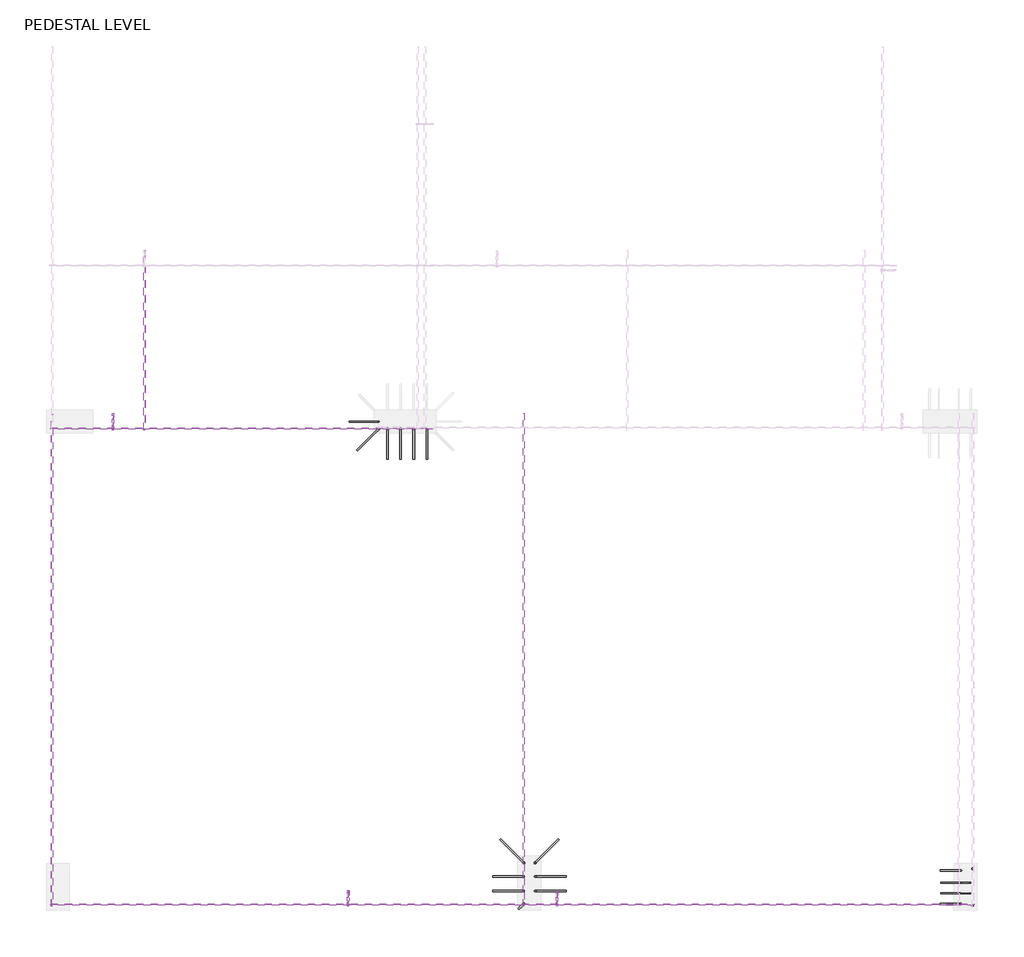
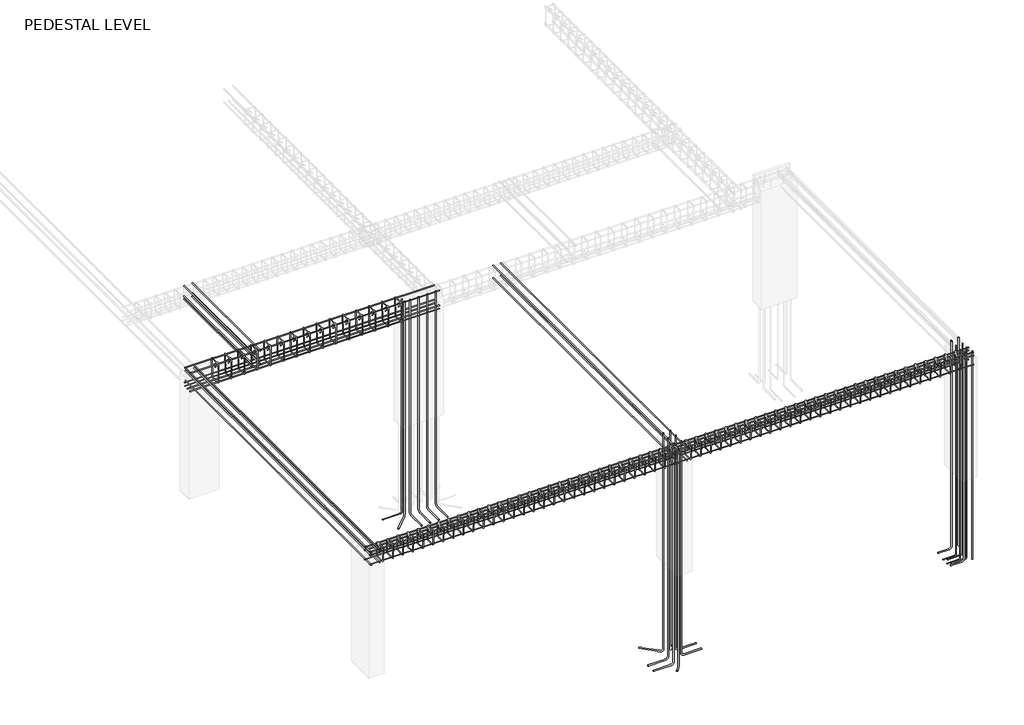
# One storey, part 2 of 8: 32 reinforcing bars.
"""IFC4 building model written with IfcOpenShell, lengths in millimetres."""

from ifc_helpers import new_model, si_unit, point, frame, origin, place, context, project, spatial, polyline, circle_curve, trimmed, segment, composite_curve, source, transform, mapped, element, save
from ifc_brep_helpers import swept_disk

model = new_model("IFC4")

# Units and contexts
model_context = context("Model", 3, world=origin())
ifc_project = project(units=[si_unit("LENGTHUNIT", "METRE", prefix="MILLI")], contexts=[model_context])

# Site, building, storey
site = spatial("IfcSite", under=ifc_project)
building = spatial("IfcBuilding", under=site)
storey = spatial("IfcBuildingStorey", under=building, Name="PEDESTAL LEVEL", Elevation=990.6)

# Reinforcing bars
placement = place(None, origin())
reinforcing_bar_shape = source(origin(), model_context, "Body", "SolidModel", [
    swept_disk(composite_curve([segment(polyline([(154656.2833793, -109544.1833171, -545.0702988), (154921.0833793, -109544.1833171, -545.0702988)]), True, "CONTINUOUS"), segment(trimmed(circle_curve(frame((154921.0833793, -109544.1833171, -505.0702988), z_axis=(0.0, -1.0, 0.0), x_axis=(0.0, 0.0, -40.00000000000006)), 40.0), [point((154921.0833793, -109544.1833171, -545.0702988))], [point((154961.0833793, -109544.1833171, -505.0702988))], True, "CARTESIAN"), True, "CONTINUOUS"), segment(polyline([(154961.0833793, -109544.1833171, -505.0702988), (154961.0833793, -109544.1833171, 2960.0)]), True, "CONTINUOUS")], self_intersect=False), 8.0),
])
element("IfcReinforcingBar", 1, at=placement, inside=storey, context=model_context, shape_type="MappedRepresentation", body=[
    mapped(reinforcing_bar_shape, transform((0.0, 0.0, 0.0), x_axis=(1.0, 0.0, 0.0), y_axis=(0.0, 1.0, 0.0), z_axis=(0.0, 0.0, 1.0))),
    mapped(reinforcing_bar_shape, transform((0.0, -142.0174604, 0.0), x_axis=(1.0, 0.0, 0.0), y_axis=(0.0, 1.0, 0.0), z_axis=(0.0, 0.0, 1.0))),
])
element("IfcReinforcingBar", 2, at=placement, inside=storey, context=model_context, shape_type="SolidModel", body=[
    swept_disk(composite_curve([segment(polyline([(154731.0324018, -109178.1177764, -511.0316783), (154937.0041414, -109384.089516, -511.0316783)]), True, "CONTINUOUS"), segment(trimmed(circle_curve(frame((154937.0041414, -109384.089516, -471.0316783), z_axis=(-0.7071067811865475, -0.7071067811865476, 0.0), x_axis=(0.0, 0.0, -40.0)), 40.0), [point((154937.0041414, -109384.089516, -511.0316783))], [point((154965.2884126, -109412.3737873, -471.0316783))], True, "CARTESIAN"), True, "CONTINUOUS"), segment(polyline([(154965.2884126, -109412.3737873, -471.0316783), (154965.2884126, -109412.3737873, 2960.0)]), True, "CONTINUOUS")], self_intersect=False), 8.0),
])
element("IfcReinforcingBar", 3, at=placement, inside=storey, context=model_context, shape_type="SolidModel", body=[
    swept_disk(composite_curve([segment(polyline([(154911.2154029, -109861.7007776, -528.1332902), (154934.3377607, -109838.5784198, -528.1332902)]), True, "CONTINUOUS"), segment(trimmed(circle_curve(frame((154934.3377607, -109838.5784198, -488.1332902), z_axis=(0.7071067811865476, -0.7071067811865476, 0.0), x_axis=(0.0, 0.0, -40.00000000000006)), 40.0), [point((154934.3377607, -109838.5784198, -528.1332902))], [point((154962.622032, -109810.2941485, -488.1332902))], True, "CARTESIAN"), True, "CONTINUOUS"), segment(polyline([(154962.622032, -109810.2941485, -488.1332902), (154962.622032, -109810.2941485, 2959.4)]), True, "CONTINUOUS")], self_intersect=False), 8.0),
])
reinforcing_bar_2_shape = source(origin(), model_context, "Body", "SolidModel", [
    swept_disk(composite_curve([segment(polyline([(155379.4630345, -109544.1833171, -443.6), (155114.6630345, -109544.1833171, -443.6)]), True, "CONTINUOUS"), segment(trimmed(circle_curve(frame((155114.6630345, -109544.1833171, -403.6), z_axis=(0.0, 1.0, 0.0), x_axis=(0.0, 0.0, -40.0)), 40.0), [point((155114.6630345, -109544.1833171, -443.6))], [point((155074.6630345, -109544.1833171, -403.6))], True, "CARTESIAN"), True, "CONTINUOUS"), segment(polyline([(155074.6630345, -109544.1833171, -403.6), (155074.6630345, -109544.1833171, 2960.0)]), True, "CONTINUOUS")], self_intersect=False), 8.0),
])
element("IfcReinforcingBar", 4, at=placement, inside=storey, context=model_context, shape_type="MappedRepresentation", body=[
    mapped(reinforcing_bar_2_shape, transform((0.0, 0.0, 0.0), x_axis=(1.0, 0.0, 0.0), y_axis=(0.0, 1.0, 0.0), z_axis=(0.0, 0.0, 1.0))),
    mapped(reinforcing_bar_2_shape, transform((0.0, -142.0174604, 0.0), x_axis=(1.0, 0.0, 0.0), y_axis=(0.0, 1.0, 0.0), z_axis=(0.0, 0.0, 1.0))),
])
element("IfcReinforcingBar", 5, at=placement, inside=storey, context=model_context, shape_type="SolidModel", body=[
    swept_disk(composite_curve([segment(polyline([(155304.7140121, -109178.1177764, -529.6040924), (155100.1944375, -109382.637351, -529.6040924)]), True, "CONTINUOUS"), segment(trimmed(circle_curve(frame((155100.1944375, -109382.637351, -489.6040924), z_axis=(-0.7071067811865475, 0.7071067811865476, 0.0), x_axis=(0.0, 0.0, -40.0)), 40.0), [point((155100.1944375, -109382.637351, -529.6040924))], [point((155071.9101663, -109410.9216222, -489.6040924))], True, "CARTESIAN"), True, "CONTINUOUS"), segment(polyline([(155071.9101663, -109410.9216222, -489.6040924), (155071.9101663, -109410.9216222, 2960.0)]), True, "CONTINUOUS")], self_intersect=False), 8.0),
])
element("IfcReinforcingBar", 6, at=placement, inside=storey, context=model_context, shape_type="SolidModel", body=[
    swept_disk(composite_curve([segment(polyline([(153542.0683747, -105141.6129875, 2960.0), (153542.0683747, -105141.6129875, -403.6)]), True, "CONTINUOUS"), segment(trimmed(circle_curve(frame((153513.7841035, -105169.8972587, -403.6), z_axis=(-0.7071067811865475, 0.7071067811865476, 0.0), x_axis=(28.28427120001288, 28.28427119999833, 0.0)), 40.0), [point((153542.0683747, -105141.6129875, -403.6))], [point((153513.7841035, -105169.8972587, -443.6))], True, "CARTESIAN"), True, "CONTINUOUS"), segment(polyline([(153513.7841035, -105169.8972587, -443.6), (153325.7544377, -105357.9269245, -443.6)]), True, "CONTINUOUS")], self_intersect=False), 8.0),
])
reinforcing_bar_3_shape = source(origin(), model_context, "Body", "SolidModel", [
    swept_disk(composite_curve([segment(polyline([(153622.3679184, -105142.4007776, 2960.0), (153622.3679184, -105142.4007776, -403.6)]), True, "CONTINUOUS"), segment(trimmed(circle_curve(frame((153622.3679184, -105182.4007776, -403.6), z_axis=(-1.0, 0.0, 0.0), x_axis=(0.0, 40.0, 0.0)), 40.0), [point((153622.3679184, -105142.4007776, -403.6))], [point((153622.3679184, -105182.4007776, -443.6))], True, "CARTESIAN"), True, "CONTINUOUS"), segment(polyline([(153622.3679184, -105182.4007776, -443.6), (153622.3679184, -105446.4942812, -443.6)]), True, "CONTINUOUS")], self_intersect=False), 8.0),
])
element("IfcReinforcingBar", 7, at=placement, inside=storey, context=model_context, shape_type="MappedRepresentation", body=[
    mapped(reinforcing_bar_3_shape, transform((0.0, 0.0, 0.0), x_axis=(1.0, 0.0, 0.0), y_axis=(0.0, 1.0, 0.0), z_axis=(0.0, 0.0, 1.0))),
    mapped(reinforcing_bar_3_shape, transform((129.6631524, 0.0, 0.0), x_axis=(1.0, 0.0, 0.0), y_axis=(0.0, 1.0, 0.0), z_axis=(0.0, 0.0, 1.0))),
    mapped(reinforcing_bar_3_shape, transform((259.3263047, 0.0, 0.0), x_axis=(1.0, 0.0, 0.0), y_axis=(0.0, 1.0, 0.0), z_axis=(0.0, 0.0, 1.0))),
    mapped(reinforcing_bar_3_shape, transform((388.9894571, 0.0, 0.0), x_axis=(1.0, 0.0, 0.0), y_axis=(0.0, 1.0, 0.0), z_axis=(0.0, 0.0, 1.0))),
])
element("IfcReinforcingBar", 8, at=placement, inside=storey, context=model_context, shape_type="SolidModel", body=[
    swept_disk(composite_curve([segment(polyline([(153537.2805846, -105076.4757776, 2960.0), (153537.2805846, -105076.4757776, -423.6)]), True, "CONTINUOUS"), segment(trimmed(circle_curve(frame((153517.2805846, -105076.4757776, -423.6), z_axis=(0.0, 1.0, 0.0), x_axis=(20.0, 0.0, 0.0)), 20.0), [point((153537.2805846, -105076.4757776, -423.6))], [point((153517.2805846, -105076.4757776, -443.6))], True, "CARTESIAN"), True, "CONTINUOUS"), segment(polyline([(153517.2805846, -105076.4757776, -443.6), (153249.1805846, -105076.4757776, -443.6)]), True, "CONTINUOUS")], self_intersect=False), 4.0),
])
reinforcing_bar_4_shape = source(origin(), model_context, "Body", "SolidModel", [
    swept_disk(composite_curve([segment(polyline([(159370.0800612, -109467.8439233, 2970.0), (159370.0800612, -109467.8439233, -330.0)]), True, "CONTINUOUS")], self_intersect=False), 8.0),
])
element("IfcReinforcingBar", 9, at=placement, inside=storey, context=model_context, shape_type="MappedRepresentation", body=[
    mapped(reinforcing_bar_4_shape, transform((0.0, 0.0, 0.0), x_axis=(1.0, 0.0, 0.0), y_axis=(0.0, 1.0, 0.0), z_axis=(0.0, 0.0, 1.0))),
    mapped(reinforcing_bar_4_shape, transform((0.0, -360.5137085, 0.0), x_axis=(1.0, 0.0, 0.0), y_axis=(0.0, 1.0, 0.0), z_axis=(0.0, 0.0, 1.0))),
])
reinforcing_bar_5_shape = source(origin(), model_context, "Body", "SolidModel", [
    swept_disk(composite_curve([segment(polyline([(159254.5094984, -109484.1870691, 2970.0), (159254.5094984, -109484.1870691, -290.0)]), True, "CONTINUOUS"), segment(trimmed(circle_curve(frame((159214.5094984, -109484.1870691, -290.0), z_axis=(0.0, 1.0, 0.0), x_axis=(40.0, 0.0, 0.0)), 40.0), [point((159254.5094984, -109484.1870691, -290.0))], [point((159214.5094984, -109484.1870691, -330.0))], True, "CARTESIAN"), True, "CONTINUOUS"), segment(polyline([(159214.5094984, -109484.1870691, -330.0), (159051.3094984, -109484.1870691, -330.0)]), True, "CONTINUOUS")], self_intersect=False), 8.0),
])
element("IfcReinforcingBar", 10, at=placement, inside=storey, context=model_context, shape_type="MappedRepresentation", body=[
    mapped(reinforcing_bar_5_shape, transform((0.0, 0.0, 0.0), x_axis=(1.0, 0.0, 0.0), y_axis=(0.0, 1.0, 0.0), z_axis=(0.0, 0.0, 1.0))),
    mapped(reinforcing_bar_5_shape, transform((0.0, -327.827417, 0.0), x_axis=(1.0, 0.0, 0.0), y_axis=(0.0, 1.0, 0.0), z_axis=(0.0, 0.0, 1.0))),
])
reinforcing_bar_6_shape = source(origin(), model_context, "Body", "SolidModel", [
    swept_disk(composite_curve([segment(polyline([(159348.801129, -109605.7653698, 2970.0), (159348.801129, -109605.7653698, -364.5307795)]), True, "CONTINUOUS"), segment(trimmed(circle_curve(frame((159328.801129, -109605.7653698, -364.5307795), z_axis=(0.0, 1.0, 0.0), x_axis=(20.0, 0.0, 0.0)), 20.0), [point((159348.801129, -109605.7653698, -364.5307795))], [point((159328.801129, -109605.7653698, -384.5307795))], True, "CARTESIAN"), True, "CONTINUOUS"), segment(polyline([(159328.801129, -109605.7653698, -384.5307795), (159122.7971827, -109605.7653698, -384.5307795)]), True, "CONTINUOUS")], self_intersect=False), 4.0),
])
element("IfcReinforcingBar", 11, at=placement, inside=storey, context=model_context, shape_type="MappedRepresentation", body=[
    mapped(reinforcing_bar_6_shape, transform((0.0, 0.0, 0.0), x_axis=(1.0, 0.0, 0.0), y_axis=(0.0, 1.0, 0.0), z_axis=(0.0, 0.0, 1.0))),
    mapped(reinforcing_bar_6_shape, transform((0.0, -103.930918, 0.0), x_axis=(1.0, 0.0, 0.0), y_axis=(0.0, 1.0, 0.0), z_axis=(0.0, 0.0, 1.0))),
])
reinforcing_bar_7_shape = source(origin(), model_context, "Body", "SolidModel", [
    swept_disk(composite_curve([segment(polyline([(159253.0952849, -109605.2805903, 2970.0), (159253.0952849, -109605.2805903, -344.9008977)]), True, "CONTINUOUS"), segment(trimmed(circle_curve(frame((159233.0952849, -109605.2805903, -344.9008977), z_axis=(0.0, 1.0, 0.0), x_axis=(20.0, 0.0, 0.0)), 20.0), [point((159253.0952849, -109605.2805903, -344.9008977))], [point((159233.0952849, -109605.2805903, -364.9008977))], True, "CARTESIAN"), True, "CONTINUOUS"), segment(polyline([(159233.0952849, -109605.2805903, -364.9008977), (159056.2452849, -109605.2805903, -364.9008977)]), True, "CONTINUOUS")], self_intersect=False), 4.0),
])
element("IfcReinforcingBar", 12, at=placement, inside=storey, context=model_context, shape_type="MappedRepresentation", body=[
    mapped(reinforcing_bar_7_shape, transform((0.0, 0.0, 0.0), x_axis=(1.0, 0.0, 0.0), y_axis=(0.0, 1.0, 0.0), z_axis=(0.0, 0.0, 1.0))),
    mapped(reinforcing_bar_7_shape, transform((0.0, -103.930918, 0.0), x_axis=(1.0, 0.0, 0.0), y_axis=(0.0, 1.0, 0.0), z_axis=(0.0, 0.0, 1.0))),
])
reinforcing_bar_8_shape = source(origin(), model_context, "Body", "SolidModel", [
    swept_disk(composite_curve([segment(polyline([(159185.8232069, -109780.5896303, 2885.7954185), (159185.8232069, -109716.2429132, 2950.1421356)]), True, "CONTINUOUS"), segment(trimmed(circle_curve(frame((159185.8232069, -109702.1007776, 2936.0), z_axis=(-1.0, 0.0, 0.0), x_axis=(0.0, -14.142135599991889, 14.142135600000074)), 20.0), [point((159185.8232069, -109716.2429132, 2950.1421356))], [point((159185.8232069, -109682.1007776, 2936.0))], True, "CARTESIAN"), True, "CONTINUOUS"), segment(polyline([(159185.8232069, -109682.1007776, 2936.0), (159185.8232069, -109682.1007776, 2749.2)]), True, "CONTINUOUS"), segment(trimmed(circle_curve(frame((159185.8232069, -109702.1007776, 2749.2), z_axis=(-1.0, 0.0, 0.0), x_axis=(0.0, 20.0, 0.0)), 20.0), [point((159185.8232069, -109682.1007776, 2749.2))], [point((159185.8232069, -109702.1007776, 2729.2))], True, "CARTESIAN"), True, "CONTINUOUS"), segment(polyline([(159185.8232069, -109702.1007776, 2729.2), (159185.8232069, -109812.7007776, 2729.2)]), True, "CONTINUOUS"), segment(trimmed(circle_curve(frame((159186.5282358, -109812.7007776, 2749.1875695), z_axis=(-0.9993784746547562, 0.0, 0.035251445314100446), x_axis=(-0.7050289000035264, 0.0, -19.987569500000063)), 20.0), [point((159185.8232069, -109812.7007776, 2729.2))], [point((159186.5282358, -109832.7007776, 2749.1875695))], True, "CARTESIAN"), True, "CONTINUOUS"), segment(polyline([(159186.5282358, -109832.7007776, 2749.1875695), (159193.118178, -109832.7007776, 2936.0124305)]), True, "CONTINUOUS"), segment(trimmed(circle_curve(frame((159193.118178, -109812.7007776, 2936.0124305), z_axis=(-0.9993784746547562, 0.0, 0.035251445314100446), x_axis=(0.0, -20.0, 0.0)), 20.0), [point((159193.118178, -109832.7007776, 2936.0124305))], [point((159193.8232069, -109812.7007776, 2956.0))], True, "CARTESIAN"), True, "CONTINUOUS"), segment(polyline([(159193.8232069, -109812.7007776, 2956.0), (159193.8232069, -109702.1007776, 2956.0)]), True, "CONTINUOUS"), segment(trimmed(circle_curve(frame((159193.8232069, -109702.1007776, 2936.0), z_axis=(-1.0, 0.0, 0.0), x_axis=(0.0, 0.0, 20.0)), 20.0), [point((159193.8232069, -109702.1007776, 2956.0))], [point((159193.8232069, -109687.958642, 2921.8578644))], True, "CARTESIAN"), True, "CONTINUOUS"), segment(polyline([(159193.8232069, -109687.958642, 2921.8578644), (159193.8232069, -109752.305359, 2857.5111473)]), True, "CONTINUOUS")], self_intersect=False), 4.0),
])
element("IfcReinforcingBar", 13, at=placement, inside=storey, context=model_context, shape_type="MappedRepresentation", body=[
    mapped(reinforcing_bar_8_shape, transform((0.0, 0.0, 0.0), x_axis=(1.0, 0.0, 0.0), y_axis=(0.0, 1.0, 0.0), z_axis=(0.0, 0.0, 1.0))),
    mapped(reinforcing_bar_8_shape, transform((-149.987037, 0.0, 0.0), x_axis=(1.0, 0.0, 0.0), y_axis=(0.0, 1.0, 0.0), z_axis=(0.0, 0.0, 1.0))),
    mapped(reinforcing_bar_8_shape, transform((-299.9740741, 0.0, 0.0), x_axis=(1.0, 0.0, 0.0), y_axis=(0.0, 1.0, 0.0), z_axis=(0.0, 0.0, 1.0))),
    mapped(reinforcing_bar_8_shape, transform((-449.9611111, 0.0, 0.0), x_axis=(1.0, 0.0, 0.0), y_axis=(0.0, 1.0, 0.0), z_axis=(0.0, 0.0, 1.0))),
    mapped(reinforcing_bar_8_shape, transform((-599.9481481, 0.0, 0.0), x_axis=(1.0, 0.0, 0.0), y_axis=(0.0, 1.0, 0.0), z_axis=(0.0, 0.0, 1.0))),
    mapped(reinforcing_bar_8_shape, transform((-749.9351852, 0.0, 0.0), x_axis=(1.0, 0.0, 0.0), y_axis=(0.0, 1.0, 0.0), z_axis=(0.0, 0.0, 1.0))),
    mapped(reinforcing_bar_8_shape, transform((-899.9222222, 0.0, 0.0), x_axis=(1.0, 0.0, 0.0), y_axis=(0.0, 1.0, 0.0), z_axis=(0.0, 0.0, 1.0))),
    mapped(reinforcing_bar_8_shape, transform((-1049.9092593, 0.0, 0.0), x_axis=(1.0, 0.0, 0.0), y_axis=(0.0, 1.0, 0.0), z_axis=(0.0, 0.0, 1.0))),
    mapped(reinforcing_bar_8_shape, transform((-1199.8962963, 0.0, 0.0), x_axis=(1.0, 0.0, 0.0), y_axis=(0.0, 1.0, 0.0), z_axis=(0.0, 0.0, 1.0))),
    mapped(reinforcing_bar_8_shape, transform((-1349.8833333, 0.0, 0.0), x_axis=(1.0, 0.0, 0.0), y_axis=(0.0, 1.0, 0.0), z_axis=(0.0, 0.0, 1.0))),
    mapped(reinforcing_bar_8_shape, transform((-1499.8703704, 0.0, 0.0), x_axis=(1.0, 0.0, 0.0), y_axis=(0.0, 1.0, 0.0), z_axis=(0.0, 0.0, 1.0))),
    mapped(reinforcing_bar_8_shape, transform((-1649.8574074, 0.0, 0.0), x_axis=(1.0, 0.0, 0.0), y_axis=(0.0, 1.0, 0.0), z_axis=(0.0, 0.0, 1.0))),
    mapped(reinforcing_bar_8_shape, transform((-1799.8444444, 0.0, 0.0), x_axis=(1.0, 0.0, 0.0), y_axis=(0.0, 1.0, 0.0), z_axis=(0.0, 0.0, 1.0))),
    mapped(reinforcing_bar_8_shape, transform((-1949.8314815, 0.0, 0.0), x_axis=(1.0, 0.0, 0.0), y_axis=(0.0, 1.0, 0.0), z_axis=(0.0, 0.0, 1.0))),
    mapped(reinforcing_bar_8_shape, transform((-2099.8185185, 0.0, 0.0), x_axis=(1.0, 0.0, 0.0), y_axis=(0.0, 1.0, 0.0), z_axis=(0.0, 0.0, 1.0))),
    mapped(reinforcing_bar_8_shape, transform((-2249.8055556, 0.0, 0.0), x_axis=(1.0, 0.0, 0.0), y_axis=(0.0, 1.0, 0.0), z_axis=(0.0, 0.0, 1.0))),
    mapped(reinforcing_bar_8_shape, transform((-2399.7925926, 0.0, 0.0), x_axis=(1.0, 0.0, 0.0), y_axis=(0.0, 1.0, 0.0), z_axis=(0.0, 0.0, 1.0))),
    mapped(reinforcing_bar_8_shape, transform((-2549.7796296, 0.0, 0.0), x_axis=(1.0, 0.0, 0.0), y_axis=(0.0, 1.0, 0.0), z_axis=(0.0, 0.0, 1.0))),
    mapped(reinforcing_bar_8_shape, transform((-2699.7666667, 0.0, 0.0), x_axis=(1.0, 0.0, 0.0), y_axis=(0.0, 1.0, 0.0), z_axis=(0.0, 0.0, 1.0))),
    mapped(reinforcing_bar_8_shape, transform((-2849.7537037, 0.0, 0.0), x_axis=(1.0, 0.0, 0.0), y_axis=(0.0, 1.0, 0.0), z_axis=(0.0, 0.0, 1.0))),
    mapped(reinforcing_bar_8_shape, transform((-2999.7407407, 0.0, 0.0), x_axis=(1.0, 0.0, 0.0), y_axis=(0.0, 1.0, 0.0), z_axis=(0.0, 0.0, 1.0))),
    mapped(reinforcing_bar_8_shape, transform((-3149.7277778, 0.0, 0.0), x_axis=(1.0, 0.0, 0.0), y_axis=(0.0, 1.0, 0.0), z_axis=(0.0, 0.0, 1.0))),
    mapped(reinforcing_bar_8_shape, transform((-3299.7148148, 0.0, 0.0), x_axis=(1.0, 0.0, 0.0), y_axis=(0.0, 1.0, 0.0), z_axis=(0.0, 0.0, 1.0))),
    mapped(reinforcing_bar_8_shape, transform((-3449.7018519, 0.0, 0.0), x_axis=(1.0, 0.0, 0.0), y_axis=(0.0, 1.0, 0.0), z_axis=(0.0, 0.0, 1.0))),
    mapped(reinforcing_bar_8_shape, transform((-3599.6888889, 0.0, 0.0), x_axis=(1.0, 0.0, 0.0), y_axis=(0.0, 1.0, 0.0), z_axis=(0.0, 0.0, 1.0))),
    mapped(reinforcing_bar_8_shape, transform((-3749.6759259, 0.0, 0.0), x_axis=(1.0, 0.0, 0.0), y_axis=(0.0, 1.0, 0.0), z_axis=(0.0, 0.0, 1.0))),
    mapped(reinforcing_bar_8_shape, transform((-3899.662963, 0.0, 0.0), x_axis=(1.0, 0.0, 0.0), y_axis=(0.0, 1.0, 0.0), z_axis=(0.0, 0.0, 1.0))),
    mapped(reinforcing_bar_8_shape, transform((-4049.65, 0.0, 0.0), x_axis=(1.0, 0.0, 0.0), y_axis=(0.0, 1.0, 0.0), z_axis=(0.0, 0.0, 1.0))),
])
reinforcing_bar_9_shape = source(origin(), model_context, "Body", "SolidModel", [
    swept_disk(composite_curve([segment(polyline([(159388.4232069, -109819.7718454, 2943.0710678), (154943.5732069, -109819.7718454, 2943.0710678)]), True, "CONTINUOUS")], self_intersect=False), 6.0),
])
element("IfcReinforcingBar", 14, at=placement, inside=storey, context=model_context, shape_type="MappedRepresentation", body=[
    mapped(reinforcing_bar_9_shape, transform((0.0, 0.0, 0.0), x_axis=(1.0, 0.0, 0.0), y_axis=(0.0, 1.0, 0.0), z_axis=(0.0, 0.0, 1.0))),
    mapped(reinforcing_bar_9_shape, transform((0.0, 124.7421356, 0.0), x_axis=(1.0, 0.0, 0.0), y_axis=(0.0, 1.0, 0.0), z_axis=(0.0, 0.0, 1.0))),
])
reinforcing_bar_10_shape = source(origin(), model_context, "Body", "SolidModel", [
    swept_disk(composite_curve([segment(polyline([(159388.4232069, -109692.1007776, 2749.2), (154943.5732069, -109692.1007776, 2749.2)]), True, "CONTINUOUS")], self_intersect=False), 6.0),
])
element("IfcReinforcingBar", 15, at=placement, inside=storey, context=model_context, shape_type="MappedRepresentation", body=[
    mapped(reinforcing_bar_10_shape, transform((0.0, 0.0, 0.0), x_axis=(1.0, 0.0, 0.0), y_axis=(0.0, 1.0, 0.0), z_axis=(0.0, 0.0, 1.0))),
    mapped(reinforcing_bar_10_shape, transform((0.0, -130.6, 0.0), x_axis=(1.0, 0.0, 0.0), y_axis=(0.0, 1.0, 0.0), z_axis=(0.0, 0.0, 1.0))),
])
reinforcing_bar_11_shape = source(origin(), model_context, "Body", "SolidModel", [
    swept_disk(composite_curve([segment(polyline([(159388.4232069, -109822.7007776, 2896.5439131), (154943.5732069, -109822.7007776, 2896.5439131)]), True, "CONTINUOUS")], self_intersect=False), 6.0),
])
element("IfcReinforcingBar", 16, at=placement, inside=storey, context=model_context, shape_type="MappedRepresentation", body=[
    mapped(reinforcing_bar_11_shape, transform((0.0, 0.0, 0.0), x_axis=(1.0, 0.0, 0.0), y_axis=(0.0, 1.0, 0.0), z_axis=(0.0, 0.0, 1.0))),
    mapped(reinforcing_bar_11_shape, transform((0.0, 130.6, 0.0), x_axis=(1.0, 0.0, 0.0), y_axis=(0.0, 1.0, 0.0), z_axis=(0.0, 0.0, 1.0))),
])
reinforcing_bar_12_shape = source(origin(), model_context, "Body", "SolidModel", [
    swept_disk(composite_curve([segment(polyline([(154899.5732069, -109780.5896303, 2885.7954185), (154899.5732069, -109716.2429132, 2950.1421356)]), True, "CONTINUOUS"), segment(trimmed(circle_curve(frame((154899.5732069, -109702.1007776, 2936.0), z_axis=(-1.0, 0.0, 0.0), x_axis=(0.0, -14.142135599991889, 14.142135600000074)), 20.0), [point((154899.5732069, -109716.2429132, 2950.1421356))], [point((154899.5732069, -109682.1007776, 2936.0))], True, "CARTESIAN"), True, "CONTINUOUS"), segment(polyline([(154899.5732069, -109682.1007776, 2936.0), (154899.5732069, -109682.1007776, 2749.2)]), True, "CONTINUOUS"), segment(trimmed(circle_curve(frame((154899.5732069, -109702.1007776, 2749.2), z_axis=(-1.0, 0.0, 0.0), x_axis=(0.0, 20.0, 0.0)), 20.0), [point((154899.5732069, -109682.1007776, 2749.2))], [point((154899.5732069, -109702.1007776, 2729.2))], True, "CARTESIAN"), True, "CONTINUOUS"), segment(polyline([(154899.5732069, -109702.1007776, 2729.2), (154899.5732069, -109812.7007776, 2729.2)]), True, "CONTINUOUS"), segment(trimmed(circle_curve(frame((154900.2782358, -109812.7007776, 2749.1875695), z_axis=(-0.9993784746547562, 0.0, 0.035251445314100446), x_axis=(-0.7050289000035264, 0.0, -19.987569500000063)), 20.0), [point((154899.5732069, -109812.7007776, 2729.2))], [point((154900.2782358, -109832.7007776, 2749.1875695))], True, "CARTESIAN"), True, "CONTINUOUS"), segment(polyline([(154900.2782358, -109832.7007776, 2749.1875695), (154906.868178, -109832.7007776, 2936.0124305)]), True, "CONTINUOUS"), segment(trimmed(circle_curve(frame((154906.868178, -109812.7007776, 2936.0124305), z_axis=(-0.9993784746547562, 0.0, 0.035251445314100446), x_axis=(0.0, -20.0, 0.0)), 20.0), [point((154906.868178, -109832.7007776, 2936.0124305))], [point((154907.5732069, -109812.7007776, 2956.0))], True, "CARTESIAN"), True, "CONTINUOUS"), segment(polyline([(154907.5732069, -109812.7007776, 2956.0), (154907.5732069, -109702.1007776, 2956.0)]), True, "CONTINUOUS"), segment(trimmed(circle_curve(frame((154907.5732069, -109702.1007776, 2936.0), z_axis=(-1.0, 0.0, 0.0), x_axis=(0.0, 0.0, 20.0)), 20.0), [point((154907.5732069, -109702.1007776, 2956.0))], [point((154907.5732069, -109687.958642, 2921.8578644))], True, "CARTESIAN"), True, "CONTINUOUS"), segment(polyline([(154907.5732069, -109687.958642, 2921.8578644), (154907.5732069, -109752.305359, 2857.5111473)]), True, "CONTINUOUS")], self_intersect=False), 4.0),
])
element("IfcReinforcingBar", 17, at=placement, inside=storey, context=model_context, shape_type="MappedRepresentation", body=[
    mapped(reinforcing_bar_12_shape, transform((0.0, 0.0, 0.0), x_axis=(1.0, 0.0, 0.0), y_axis=(0.0, 1.0, 0.0), z_axis=(0.0, 0.0, 1.0))),
    mapped(reinforcing_bar_12_shape, transform((-151.4672414, 0.0, 0.0), x_axis=(1.0, 0.0, 0.0), y_axis=(0.0, 1.0, 0.0), z_axis=(0.0, 0.0, 1.0))),
    mapped(reinforcing_bar_12_shape, transform((-302.9344828, 0.0, 0.0), x_axis=(1.0, 0.0, 0.0), y_axis=(0.0, 1.0, 0.0), z_axis=(0.0, 0.0, 1.0))),
    mapped(reinforcing_bar_12_shape, transform((-454.4017241, 0.0, 0.0), x_axis=(1.0, 0.0, 0.0), y_axis=(0.0, 1.0, 0.0), z_axis=(0.0, 0.0, 1.0))),
    mapped(reinforcing_bar_12_shape, transform((-605.8689655, 0.0, 0.0), x_axis=(1.0, 0.0, 0.0), y_axis=(0.0, 1.0, 0.0), z_axis=(0.0, 0.0, 1.0))),
    mapped(reinforcing_bar_12_shape, transform((-757.3362069, 0.0, 0.0), x_axis=(1.0, 0.0, 0.0), y_axis=(0.0, 1.0, 0.0), z_axis=(0.0, 0.0, 1.0))),
    mapped(reinforcing_bar_12_shape, transform((-908.8034483, 0.0, 0.0), x_axis=(1.0, 0.0, 0.0), y_axis=(0.0, 1.0, 0.0), z_axis=(0.0, 0.0, 1.0))),
    mapped(reinforcing_bar_12_shape, transform((-1060.2706897, 0.0, 0.0), x_axis=(1.0, 0.0, 0.0), y_axis=(0.0, 1.0, 0.0), z_axis=(0.0, 0.0, 1.0))),
    mapped(reinforcing_bar_12_shape, transform((-1211.737931, 0.0, 0.0), x_axis=(1.0, 0.0, 0.0), y_axis=(0.0, 1.0, 0.0), z_axis=(0.0, 0.0, 1.0))),
    mapped(reinforcing_bar_12_shape, transform((-1363.2051724, 0.0, 0.0), x_axis=(1.0, 0.0, 0.0), y_axis=(0.0, 1.0, 0.0), z_axis=(0.0, 0.0, 1.0))),
    mapped(reinforcing_bar_12_shape, transform((-1514.6724138, 0.0, 0.0), x_axis=(1.0, 0.0, 0.0), y_axis=(0.0, 1.0, 0.0), z_axis=(0.0, 0.0, 1.0))),
    mapped(reinforcing_bar_12_shape, transform((-1666.1396552, 0.0, 0.0), x_axis=(1.0, 0.0, 0.0), y_axis=(0.0, 1.0, 0.0), z_axis=(0.0, 0.0, 1.0))),
    mapped(reinforcing_bar_12_shape, transform((-1817.6068966, 0.0, 0.0), x_axis=(1.0, 0.0, 0.0), y_axis=(0.0, 1.0, 0.0), z_axis=(0.0, 0.0, 1.0))),
    mapped(reinforcing_bar_12_shape, transform((-1969.0741379, 0.0, 0.0), x_axis=(1.0, 0.0, 0.0), y_axis=(0.0, 1.0, 0.0), z_axis=(0.0, 0.0, 1.0))),
    mapped(reinforcing_bar_12_shape, transform((-2120.5413793, 0.0, 0.0), x_axis=(1.0, 0.0, 0.0), y_axis=(0.0, 1.0, 0.0), z_axis=(0.0, 0.0, 1.0))),
    mapped(reinforcing_bar_12_shape, transform((-2272.0086207, 0.0, 0.0), x_axis=(1.0, 0.0, 0.0), y_axis=(0.0, 1.0, 0.0), z_axis=(0.0, 0.0, 1.0))),
    mapped(reinforcing_bar_12_shape, transform((-2423.4758621, 0.0, 0.0), x_axis=(1.0, 0.0, 0.0), y_axis=(0.0, 1.0, 0.0), z_axis=(0.0, 0.0, 1.0))),
    mapped(reinforcing_bar_12_shape, transform((-2574.9431034, 0.0, 0.0), x_axis=(1.0, 0.0, 0.0), y_axis=(0.0, 1.0, 0.0), z_axis=(0.0, 0.0, 1.0))),
    mapped(reinforcing_bar_12_shape, transform((-2726.4103448, 0.0, 0.0), x_axis=(1.0, 0.0, 0.0), y_axis=(0.0, 1.0, 0.0), z_axis=(0.0, 0.0, 1.0))),
    mapped(reinforcing_bar_12_shape, transform((-2877.8775862, 0.0, 0.0), x_axis=(1.0, 0.0, 0.0), y_axis=(0.0, 1.0, 0.0), z_axis=(0.0, 0.0, 1.0))),
    mapped(reinforcing_bar_12_shape, transform((-3029.3448276, 0.0, 0.0), x_axis=(1.0, 0.0, 0.0), y_axis=(0.0, 1.0, 0.0), z_axis=(0.0, 0.0, 1.0))),
    mapped(reinforcing_bar_12_shape, transform((-3180.812069, 0.0, 0.0), x_axis=(1.0, 0.0, 0.0), y_axis=(0.0, 1.0, 0.0), z_axis=(0.0, 0.0, 1.0))),
    mapped(reinforcing_bar_12_shape, transform((-3332.2793103, 0.0, 0.0), x_axis=(1.0, 0.0, 0.0), y_axis=(0.0, 1.0, 0.0), z_axis=(0.0, 0.0, 1.0))),
    mapped(reinforcing_bar_12_shape, transform((-3483.7465517, 0.0, 0.0), x_axis=(1.0, 0.0, 0.0), y_axis=(0.0, 1.0, 0.0), z_axis=(0.0, 0.0, 1.0))),
    mapped(reinforcing_bar_12_shape, transform((-3635.2137931, 0.0, 0.0), x_axis=(1.0, 0.0, 0.0), y_axis=(0.0, 1.0, 0.0), z_axis=(0.0, 0.0, 1.0))),
    mapped(reinforcing_bar_12_shape, transform((-3786.6810345, 0.0, 0.0), x_axis=(1.0, 0.0, 0.0), y_axis=(0.0, 1.0, 0.0), z_axis=(0.0, 0.0, 1.0))),
    mapped(reinforcing_bar_12_shape, transform((-3938.1482759, 0.0, 0.0), x_axis=(1.0, 0.0, 0.0), y_axis=(0.0, 1.0, 0.0), z_axis=(0.0, 0.0, 1.0))),
    mapped(reinforcing_bar_12_shape, transform((-4089.6155172, 0.0, 0.0), x_axis=(1.0, 0.0, 0.0), y_axis=(0.0, 1.0, 0.0), z_axis=(0.0, 0.0, 1.0))),
    mapped(reinforcing_bar_12_shape, transform((-4241.0827586, 0.0, 0.0), x_axis=(1.0, 0.0, 0.0), y_axis=(0.0, 1.0, 0.0), z_axis=(0.0, 0.0, 1.0))),
    mapped(reinforcing_bar_12_shape, transform((-4392.55, 0.0, 0.0), x_axis=(1.0, 0.0, 0.0), y_axis=(0.0, 1.0, 0.0), z_axis=(0.0, 0.0, 1.0))),
])
reinforcing_bar_13_shape = source(origin(), model_context, "Body", "SolidModel", [
    swept_disk(composite_curve([segment(polyline([(154943.5732069, -109819.7718454, 2943.0710678), (150314.4232069, -109819.7718454, 2943.0710678)]), True, "CONTINUOUS")], self_intersect=False), 6.0),
])
element("IfcReinforcingBar", 18, at=placement, inside=storey, context=model_context, shape_type="MappedRepresentation", body=[
    mapped(reinforcing_bar_13_shape, transform((0.0, 0.0, 0.0), x_axis=(1.0, 0.0, 0.0), y_axis=(0.0, 1.0, 0.0), z_axis=(0.0, 0.0, 1.0))),
    mapped(reinforcing_bar_13_shape, transform((0.0, 124.7421356, 0.0), x_axis=(1.0, 0.0, 0.0), y_axis=(0.0, 1.0, 0.0), z_axis=(0.0, 0.0, 1.0))),
])
reinforcing_bar_14_shape = source(origin(), model_context, "Body", "SolidModel", [
    swept_disk(composite_curve([segment(polyline([(154943.5732069, -109692.1007776, 2749.2), (150314.4232069, -109692.1007776, 2749.2)]), True, "CONTINUOUS")], self_intersect=False), 6.0),
])
element("IfcReinforcingBar", 19, at=placement, inside=storey, context=model_context, shape_type="MappedRepresentation", body=[
    mapped(reinforcing_bar_14_shape, transform((0.0, 0.0, 0.0), x_axis=(1.0, 0.0, 0.0), y_axis=(0.0, 1.0, 0.0), z_axis=(0.0, 0.0, 1.0))),
    mapped(reinforcing_bar_14_shape, transform((0.0, -130.6, 0.0), x_axis=(1.0, 0.0, 0.0), y_axis=(0.0, 1.0, 0.0), z_axis=(0.0, 0.0, 1.0))),
])
reinforcing_bar_15_shape = source(origin(), model_context, "Body", "SolidModel", [
    swept_disk(composite_curve([segment(polyline([(154943.5732069, -109822.7007776, 2896.5439131), (150314.4232069, -109822.7007776, 2896.5439131)]), True, "CONTINUOUS")], self_intersect=False), 6.0),
])
element("IfcReinforcingBar", 20, at=placement, inside=storey, context=model_context, shape_type="MappedRepresentation", body=[
    mapped(reinforcing_bar_15_shape, transform((0.0, 0.0, 0.0), x_axis=(1.0, 0.0, 0.0), y_axis=(0.0, 1.0, 0.0), z_axis=(0.0, 0.0, 1.0))),
    mapped(reinforcing_bar_15_shape, transform((0.0, 130.6, 0.0), x_axis=(1.0, 0.0, 0.0), y_axis=(0.0, 1.0, 0.0), z_axis=(0.0, 0.0, 1.0))),
])
reinforcing_bar_16_shape = source(origin(), model_context, "Body", "SolidModel", [
    swept_disk(composite_curve([segment(polyline([(150456.0942747, -105001.8007776, 2943.0710678), (150456.0942747, -109836.7007776, 2943.0710678)]), True, "CONTINUOUS")], self_intersect=False), 6.0),
])
element("IfcReinforcingBar", 21, at=placement, inside=storey, context=model_context, shape_type="MappedRepresentation", body=[
    mapped(reinforcing_bar_16_shape, transform((0.0, 0.0, 0.0), x_axis=(1.0, 0.0, 0.0), y_axis=(0.0, 1.0, 0.0), z_axis=(0.0, 0.0, 1.0))),
    mapped(reinforcing_bar_16_shape, transform((-124.6879758, 0.0, 0.0), x_axis=(1.0, 0.0, 0.0), y_axis=(0.0, 1.0, 0.0), z_axis=(0.0, 0.0, 1.0))),
])
reinforcing_bar_17_shape = source(origin(), model_context, "Body", "SolidModel", [
    swept_disk(composite_curve([segment(polyline([(150331.3521391, -105001.8007776, 2742.1289322), (150331.3521391, -109836.7007776, 2742.1289322)]), True, "CONTINUOUS")], self_intersect=False), 6.0),
])
element("IfcReinforcingBar", 22, at=placement, inside=storey, context=model_context, shape_type="MappedRepresentation", body=[
    mapped(reinforcing_bar_17_shape, transform((0.0, 0.0, 0.0), x_axis=(1.0, 0.0, 0.0), y_axis=(0.0, 1.0, 0.0), z_axis=(0.0, 0.0, 1.0))),
    mapped(reinforcing_bar_17_shape, transform((124.7421356, 0.0, 0.0), x_axis=(1.0, 0.0, 0.0), y_axis=(0.0, 1.0, 0.0), z_axis=(0.0, 0.0, 1.0))),
])
reinforcing_bar_18_shape = source(origin(), model_context, "Body", "SolidModel", [
    swept_disk(composite_curve([segment(polyline([(150328.4232069, -105001.8007776, 2899.6682247), (150328.4232069, -109836.7007776, 2899.6682247)]), True, "CONTINUOUS")], self_intersect=False), 6.0),
])
element("IfcReinforcingBar", 23, at=placement, inside=storey, context=model_context, shape_type="MappedRepresentation", body=[
    mapped(reinforcing_bar_18_shape, transform((0.0, 0.0, 0.0), x_axis=(1.0, 0.0, 0.0), y_axis=(0.0, 1.0, 0.0), z_axis=(0.0, 0.0, 1.0))),
    mapped(reinforcing_bar_18_shape, transform((128.6, 0.0, 0.0), x_axis=(1.0, 0.0, 0.0), y_axis=(0.0, 1.0, 0.0), z_axis=(0.0, 0.0, 1.0))),
])
reinforcing_bar_19_shape = source(origin(), model_context, "Body", "SolidModel", [
    swept_disk(composite_curve([segment(polyline([(151361.5090307, -103391.6007776, 2953.0710678), (151361.5090307, -105160.4007776, 2953.0710678)]), True, "CONTINUOUS")], self_intersect=False), 6.0),
])
element("IfcReinforcingBar", 24, at=placement, inside=storey, context=model_context, shape_type="MappedRepresentation", body=[
    mapped(reinforcing_bar_19_shape, transform((0.0, 0.0, 0.0), x_axis=(1.0, 0.0, 0.0), y_axis=(0.0, 1.0, 0.0), z_axis=(0.0, 0.0, 1.0))),
    mapped(reinforcing_bar_19_shape, transform((-124.7421356, 0.0, 0.0), x_axis=(1.0, 0.0, 0.0), y_axis=(0.0, 1.0, 0.0), z_axis=(0.0, 0.0, 1.0))),
])
reinforcing_bar_20_shape = source(origin(), model_context, "Body", "SolidModel", [
    swept_disk(composite_curve([segment(polyline([(151236.766895, -103391.6007776, 2742.1289322), (151236.766895, -105160.4007776, 2742.1289322)]), True, "CONTINUOUS")], self_intersect=False), 6.0),
])
element("IfcReinforcingBar", 25, at=placement, inside=storey, context=model_context, shape_type="MappedRepresentation", body=[
    mapped(reinforcing_bar_20_shape, transform((0.0, 0.0, 0.0), x_axis=(1.0, 0.0, 0.0), y_axis=(0.0, 1.0, 0.0), z_axis=(0.0, 0.0, 1.0))),
    mapped(reinforcing_bar_20_shape, transform((124.7421356, 0.0, 0.0), x_axis=(1.0, 0.0, 0.0), y_axis=(0.0, 1.0, 0.0), z_axis=(0.0, 0.0, 1.0))),
])
reinforcing_bar_21_shape = source(origin(), model_context, "Body", "SolidModel", [
    swept_disk(composite_curve([segment(polyline([(151233.8379628, -103391.6007776, 2791.7182247), (151233.8379628, -105160.4007776, 2791.7182247)]), True, "CONTINUOUS")], self_intersect=False), 6.0),
])
element("IfcReinforcingBar", 26, at=placement, inside=storey, context=model_context, shape_type="MappedRepresentation", body=[
    mapped(reinforcing_bar_21_shape, transform((0.0, 0.0, 0.0), x_axis=(1.0, 0.0, 0.0), y_axis=(0.0, 1.0, 0.0), z_axis=(0.0, 0.0, 1.0))),
    mapped(reinforcing_bar_21_shape, transform((127.6710678, 0.0, 0.0), x_axis=(1.0, 0.0, 0.0), y_axis=(0.0, 1.0, 0.0), z_axis=(0.0, 0.0, 1.0))),
])
reinforcing_bar_22_shape = source(origin(), model_context, "Body", "SolidModel", [
    swept_disk(composite_curve([segment(polyline([(150735.6232069, -105057.9119249, 2895.7954185), (150735.6232069, -105122.258642, 2960.1421356)]), True, "CONTINUOUS"), segment(trimmed(circle_curve(frame((150735.6232069, -105136.4007776, 2946.0), z_axis=(1.0, 0.0, 0.0), x_axis=(0.0, 14.14213560000644, 14.142135600000074)), 20.0), [point((150735.6232069, -105122.258642, 2960.1421356))], [point((150735.6232069, -105156.4007776, 2946.0))], True, "CARTESIAN"), True, "CONTINUOUS"), segment(polyline([(150735.6232069, -105156.4007776, 2946.0), (150735.6232069, -105156.4007776, 2673.0)]), True, "CONTINUOUS"), segment(trimmed(circle_curve(frame((150735.6232069, -105136.4007776, 2673.0), z_axis=(1.0, 0.0, 0.0), x_axis=(0.0, -20.0, 0.0)), 20.0), [point((150735.6232069, -105156.4007776, 2673.0))], [point((150735.6232069, -105136.4007776, 2653.0))], True, "CARTESIAN"), True, "CONTINUOUS"), segment(polyline([(150735.6232069, -105136.4007776, 2653.0), (150735.6232069, -105015.8007776, 2653.0)]), True, "CONTINUOUS"), segment(trimmed(circle_curve(frame((150735.1121917, -105015.8007776, 2672.9934705), z_axis=(0.9996735260122956, 0.0, 0.025550761048237572), x_axis=(0.511015199997928, 0.0, -19.993470500000058)), 20.0), [point((150735.6232069, -105015.8007776, 2653.0))], [point((150735.1121917, -104995.8007776, 2672.9934705))], True, "CARTESIAN"), True, "CONTINUOUS"), segment(polyline([(150735.1121917, -104995.8007776, 2672.9934705), (150728.1342222, -104995.8007776, 2946.0065295)]), True, "CONTINUOUS"), segment(trimmed(circle_curve(frame((150728.1342222, -105015.8007776, 2946.0065295), z_axis=(0.9996735260122956, 0.0, 0.025550761048237572), x_axis=(0.0, 20.0, 0.0)), 20.0), [point((150728.1342222, -104995.8007776, 2946.0065295))], [point((150727.6232069, -105015.8007776, 2966.0))], True, "CARTESIAN"), True, "CONTINUOUS"), segment(polyline([(150727.6232069, -105015.8007776, 2966.0), (150727.6232069, -105136.4007776, 2966.0)]), True, "CONTINUOUS"), segment(trimmed(circle_curve(frame((150727.6232069, -105136.4007776, 2946.0), z_axis=(1.0, 0.0, 0.0), x_axis=(0.0, 0.0, 20.0)), 20.0), [point((150727.6232069, -105136.4007776, 2966.0))], [point((150727.6232069, -105150.5429132, 2931.8578644))], True, "CARTESIAN"), True, "CONTINUOUS"), segment(polyline([(150727.6232069, -105150.5429132, 2931.8578644), (150727.6232069, -105086.1961961, 2867.5111473)]), True, "CONTINUOUS")], self_intersect=False), 4.0),
])
element("IfcReinforcingBar", 27, at=placement, inside=storey, context=model_context, shape_type="MappedRepresentation", body=[
    mapped(reinforcing_bar_22_shape, transform((0.0, 0.0, 0.0), x_axis=(1.0, 0.0, 0.0), y_axis=(0.0, 1.0, 0.0), z_axis=(0.0, 0.0, 1.0))),
    mapped(reinforcing_bar_22_shape, transform((196.6898127, 0.0, 0.0), x_axis=(1.0, 0.0, 0.0), y_axis=(0.0, 1.0, 0.0), z_axis=(0.0, 0.0, 1.0))),
    mapped(reinforcing_bar_22_shape, transform((393.3796254, 0.0, 0.0), x_axis=(1.0, 0.0, 0.0), y_axis=(0.0, 1.0, 0.0), z_axis=(0.0, 0.0, 1.0))),
    mapped(reinforcing_bar_22_shape, transform((590.0694381, 0.0, 0.0), x_axis=(1.0, 0.0, 0.0), y_axis=(0.0, 1.0, 0.0), z_axis=(0.0, 0.0, 1.0))),
    mapped(reinforcing_bar_22_shape, transform((786.7592508, 0.0, 0.0), x_axis=(1.0, 0.0, 0.0), y_axis=(0.0, 1.0, 0.0), z_axis=(0.0, 0.0, 1.0))),
    mapped(reinforcing_bar_22_shape, transform((983.4490634, 0.0, 0.0), x_axis=(1.0, 0.0, 0.0), y_axis=(0.0, 1.0, 0.0), z_axis=(0.0, 0.0, 1.0))),
    mapped(reinforcing_bar_22_shape, transform((1180.1388761, 0.0, 0.0), x_axis=(1.0, 0.0, 0.0), y_axis=(0.0, 1.0, 0.0), z_axis=(0.0, 0.0, 1.0))),
    mapped(reinforcing_bar_22_shape, transform((1376.8286888, 0.0, 0.0), x_axis=(1.0, 0.0, 0.0), y_axis=(0.0, 1.0, 0.0), z_axis=(0.0, 0.0, 1.0))),
    mapped(reinforcing_bar_22_shape, transform((1573.5185015, 0.0, 0.0), x_axis=(1.0, 0.0, 0.0), y_axis=(0.0, 1.0, 0.0), z_axis=(0.0, 0.0, 1.0))),
    mapped(reinforcing_bar_22_shape, transform((1770.2083142, 0.0, 0.0), x_axis=(1.0, 0.0, 0.0), y_axis=(0.0, 1.0, 0.0), z_axis=(0.0, 0.0, 1.0))),
    mapped(reinforcing_bar_22_shape, transform((1966.8981269, 0.0, 0.0), x_axis=(1.0, 0.0, 0.0), y_axis=(0.0, 1.0, 0.0), z_axis=(0.0, 0.0, 1.0))),
    mapped(reinforcing_bar_22_shape, transform((2163.5879396, 0.0, 0.0), x_axis=(1.0, 0.0, 0.0), y_axis=(0.0, 1.0, 0.0), z_axis=(0.0, 0.0, 1.0))),
    mapped(reinforcing_bar_22_shape, transform((2360.2777523, 0.0, 0.0), x_axis=(1.0, 0.0, 0.0), y_axis=(0.0, 1.0, 0.0), z_axis=(0.0, 0.0, 1.0))),
    mapped(reinforcing_bar_22_shape, transform((2556.967565, 0.0, 0.0), x_axis=(1.0, 0.0, 0.0), y_axis=(0.0, 1.0, 0.0), z_axis=(0.0, 0.0, 1.0))),
    mapped(reinforcing_bar_22_shape, transform((2753.6573776, 0.0, 0.0), x_axis=(1.0, 0.0, 0.0), y_axis=(0.0, 1.0, 0.0), z_axis=(0.0, 0.0, 1.0))),
])
reinforcing_bar_23_shape = source(origin(), model_context, "Body", "SolidModel", [
    swept_disk(composite_curve([segment(polyline([(150314.4232069, -105008.7297098, 2953.0710678), (154062.8805846, -105008.7297098, 2953.0710678)]), True, "CONTINUOUS")], self_intersect=False), 6.0),
])
element("IfcReinforcingBar", 28, at=placement, inside=storey, context=model_context, shape_type="MappedRepresentation", body=[
    mapped(reinforcing_bar_23_shape, transform((0.0, 0.0, 0.0), x_axis=(1.0, 0.0, 0.0), y_axis=(0.0, 1.0, 0.0), z_axis=(0.0, 0.0, 1.0))),
    mapped(reinforcing_bar_23_shape, transform((0.0, -134.7421356, 0.0), x_axis=(1.0, 0.0, 0.0), y_axis=(0.0, 1.0, 0.0), z_axis=(0.0, 0.0, 1.0))),
])
reinforcing_bar_24_shape = source(origin(), model_context, "Body", "SolidModel", [
    swept_disk(composite_curve([segment(polyline([(150314.4232069, -105143.4718454, 2665.9289322), (154062.8805846, -105143.4718454, 2665.9289322)]), True, "CONTINUOUS")], self_intersect=False), 6.0),
])
element("IfcReinforcingBar", 29, at=placement, inside=storey, context=model_context, shape_type="MappedRepresentation", body=[
    mapped(reinforcing_bar_24_shape, transform((0.0, 0.0, 0.0), x_axis=(1.0, 0.0, 0.0), y_axis=(0.0, 1.0, 0.0), z_axis=(0.0, 0.0, 1.0))),
    mapped(reinforcing_bar_24_shape, transform((0.0, 67.3710678, 0.0), x_axis=(1.0, 0.0, 0.0), y_axis=(0.0, 1.0, 0.0), z_axis=(0.0, 0.0, 1.0))),
    mapped(reinforcing_bar_24_shape, transform((0.0, 134.7421356, 0.0), x_axis=(1.0, 0.0, 0.0), y_axis=(0.0, 1.0, 0.0), z_axis=(0.0, 0.0, 1.0))),
])
reinforcing_bar_25_shape = source(origin(), model_context, "Body", "SolidModel", [
    swept_disk(composite_curve([segment(polyline([(150314.4232069, -105144.9400027, 2719.5525215), (154062.8805846, -105144.9400027, 2719.5525215)]), True, "CONTINUOUS")], self_intersect=False), 6.0),
])
element("IfcReinforcingBar", 30, at=placement, inside=storey, context=model_context, shape_type="MappedRepresentation", body=[
    mapped(reinforcing_bar_25_shape, transform((0.0, 0.0, 0.0), x_axis=(1.0, 0.0, 0.0), y_axis=(0.0, 1.0, 0.0), z_axis=(0.0, 0.0, 1.0))),
    mapped(reinforcing_bar_25_shape, transform((0.0, 138.7267251, 0.0), x_axis=(1.0, 0.0, 0.0), y_axis=(0.0, 1.0, 0.0), z_axis=(0.0, 0.0, 1.0))),
])
reinforcing_bar_26_shape = source(origin(), model_context, "Body", "SolidModel", [
    swept_disk(composite_curve([segment(polyline([(154960.5021391, -104991.8007776, 2943.0710678), (154960.5021391, -109836.7007776, 2943.0710678)]), True, "CONTINUOUS")], self_intersect=False), 6.0),
])
element("IfcReinforcingBar", 31, at=placement, inside=storey, context=model_context, shape_type="MappedRepresentation", body=[
    mapped(reinforcing_bar_26_shape, transform((0.0, 0.0, 0.0), x_axis=(1.0, 0.0, 0.0), y_axis=(0.0, 1.0, 0.0), z_axis=(0.0, 0.0, 1.0))),
    mapped(reinforcing_bar_26_shape, transform((114.8635059, 0.0, 0.0), x_axis=(1.0, 0.0, 0.0), y_axis=(0.0, 1.0, 0.0), z_axis=(0.0, 0.0, 1.0))),
])
reinforcing_bar_27_shape = source(origin(), model_context, "Body", "SolidModel", [
    swept_disk(composite_curve([segment(polyline([(154960.5021391, -104991.8007776, 2742.1289322), (154960.5021391, -109836.7007776, 2742.1289322)]), True, "CONTINUOUS")], self_intersect=False), 6.0),
])
element("IfcReinforcingBar", 32, at=placement, inside=storey, context=model_context, shape_type="MappedRepresentation", body=[
    mapped(reinforcing_bar_27_shape, transform((0.0, 0.0, 0.0), x_axis=(1.0, 0.0, 0.0), y_axis=(0.0, 1.0, 0.0), z_axis=(0.0, 0.0, 1.0))),
    mapped(reinforcing_bar_27_shape, transform((114.7421356, 0.0, 0.0), x_axis=(1.0, 0.0, 0.0), y_axis=(0.0, 1.0, 0.0), z_axis=(0.0, 0.0, 1.0))),
])

save(model, "model.ifc")

# Revit data of these elements
# Elements 1, 2, 3, 4, 5, 6, 7, 8, 9, 10, 11, 12, 13, 14, 15, 16, 17, 18, 19, 20, 21, 22, 23, 24, 25, 26, 27, 28, 29, 30, 31, 32 (IfcReinforcingBar)
#   Phase Created = New Construction
